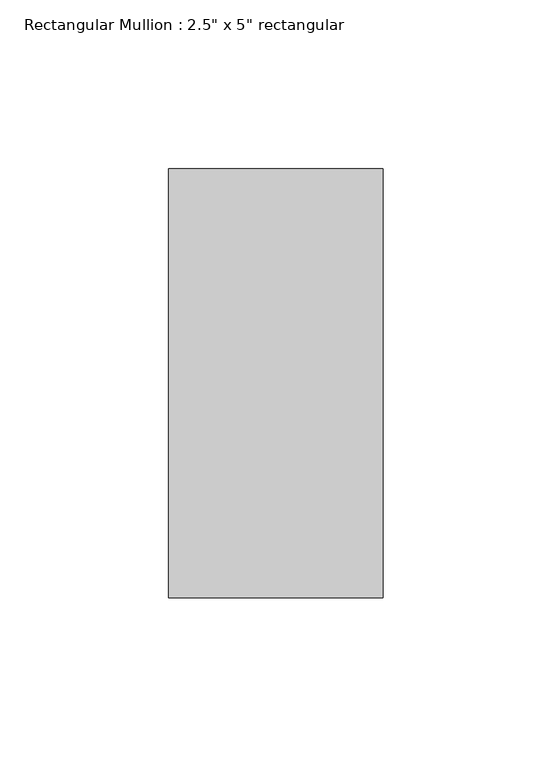
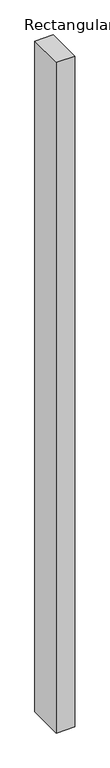
"""IFC4 building model written with IfcOpenShell, lengths in millimetres: member geometry."""

from ifc_helpers import new_model, si_unit, frame, origin, place, context, project, spatial, polyline, outline, extrude, source, transform, mapped, element, save


def member_89a537c7(model_context):
    return source(origin(), model_context, "Body", "SweptSolid", [
        extrude(outline(polyline([(31.75, 63.5), (31.75, -63.5), (-31.75, -63.5), (-31.75, 63.5), (31.75, 63.5)])), frame((0.0, 0.0, -2445.7520936), z_axis=(0.0, 0.0, 1.0), x_axis=(1.0, 0.0, 0.0)), (0.0, 0.0, 1.0), 2445.7520936),
    ])


if __name__ == "__main__":
    model = new_model("IFC4")
    model_context = context("Model", 3, world=origin())
    ifc_project = project(units=[si_unit("LENGTHUNIT", "METRE", prefix="MILLI")], contexts=[model_context])
    site = spatial("IfcSite", under=ifc_project)
    building = spatial("IfcBuilding", under=site)
    placement = place(None, origin())
    member_shape = member_89a537c7(model_context)
    element("IfcMember", 1, ObjectType="Rectangular Mullion : 2.5\" x 5\" rectangular", at=placement, inside=building, context=model_context, shape_type="MappedRepresentation", body=[
        mapped(member_shape, transform((0.0, 0.0, 0.0), x_axis=(1.0, 0.0, 0.0), y_axis=(0.0, 1.0, 0.0), z_axis=(0.0, 0.0, 1.0))),
    ])
    save(model, "model.ifc")

# Revit data of these elements
# Type "Rectangular Mullion : 2.5\" x 5\" rectangular"
#   built-in parameter 1007304 = 0.416667 (stored number, unit not read)
#   built-in parameter 1007301 = 0.104167 (stored number, unit not read)
#   built-in parameter 1007300 = 0.104167 (stored number, unit not read)
# Element 1 (IfcMember, "Rectangular Mullion : 2.5\" x 5\" rectangular")
#   Materials on its faces: "Aluminum"
# Materials
#   "Aluminum": class "Metal", colour RGB 247 247 247, transparency 0, Description = "Aluminum 6061", Cost = 0
